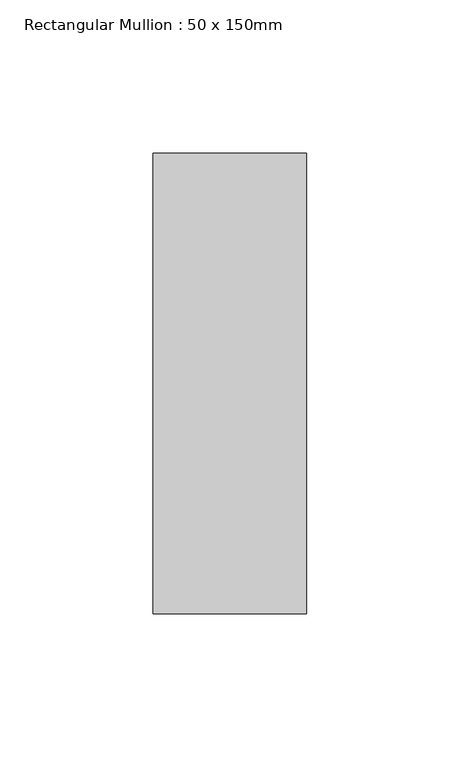
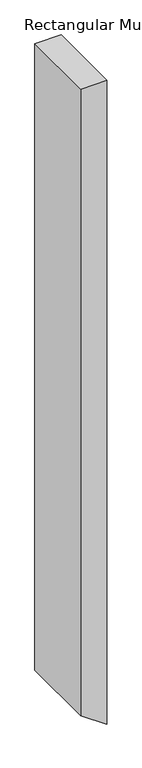
"""IFC4 building model written with IfcOpenShell, lengths in millimetres: member geometry, Rectangular Mullion : 50 x 150mm."""

from ifc_helpers import new_model, si_unit, frame, origin, place, context, project, spatial, polyline, outline, extrude, source, transform, mapped, element, save


def rectangular_mullion_50_x_150mm_bef26404(model_context):
    return source(origin(), model_context, "Body", "SweptSolid", [
        extrude(outline(polyline([(0.0, 25.0), (0.0, -25.0), (-1255.8328815, -25.0), (-1290.8432584, 25.0), (0.0, 25.0)])), frame((0.0, -75.0, 0.0), z_axis=(0.0, 1.0, 0.0), x_axis=(0.0, 0.0, 1.0)), (0.0, 0.0, 1.0), 150.0),
    ])


if __name__ == "__main__":
    model = new_model("IFC4")
    model_context = context("Model", 3, world=origin())
    ifc_project = project(units=[si_unit("LENGTHUNIT", "METRE", prefix="MILLI")], contexts=[model_context])
    site = spatial("IfcSite", under=ifc_project)
    building = spatial("IfcBuilding", under=site)
    placement = place(None, origin())
    rectangular_mullion_50_x_150mm_shape = rectangular_mullion_50_x_150mm_bef26404(model_context)
    element("IfcMember", 1, ObjectType="Rectangular Mullion : 50 x 150mm", at=placement, inside=building, context=model_context, shape_type="MappedRepresentation", body=[
        mapped(rectangular_mullion_50_x_150mm_shape, transform((0.0, 0.0, 0.0), x_axis=(1.0, 0.0, 0.0), y_axis=(0.0, 1.0, 0.0), z_axis=(0.0, 0.0, 1.0))),
    ])
    save(model, "model.ifc")

# Revit data of these elements
# Type "Rectangular Mullion : 50 x 150mm"
#   built-in parameter 1007304 = 0.492126 (stored number, unit not read)
#   built-in parameter 1007301 = 0.082021 (stored number, unit not read)
#   built-in parameter 1007300 = 0.082021 (stored number, unit not read)
# Element 1 (IfcMember, "Rectangular Mullion : 50 x 150mm")
#   Materials on its faces: "Aluminium"
# Materials
#   "Aluminium": class "Metal", colour RGB 247 247 247, transparency 0, Description = "Aluminium 6061", Cost = 0
